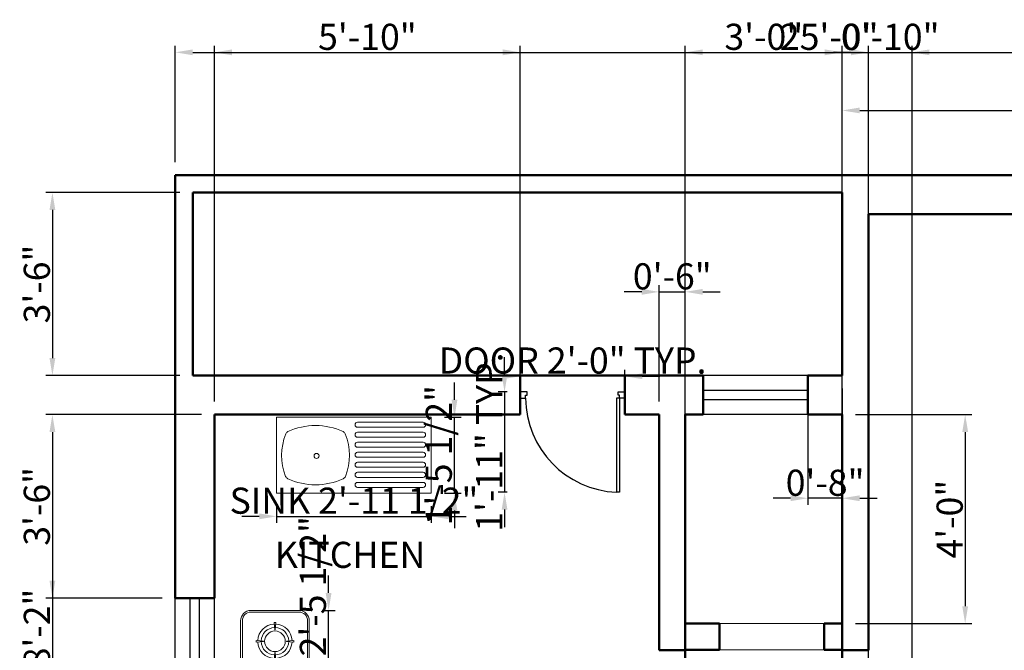
# Model space of a CAD drawing. Units: inches. Extents: x 749 to 1130, y 885 to 1490.
# Tile 4 of 5: x 754 to 980, y 1345 to 1490. Entities that reach past the tile are written whole.
import ezdxf

# ---------------------------------------------------------------- set-up
doc = ezdxf.new("R2010")
doc.units = ezdxf.units.IN
doc.header["$MEASUREMENT"] = 0
for name, color, linetype, lineweight in [('A-ANNO-DIMS', 2, 'Continuous', 18), ('A-AREA-IDEN', 7, 'Continuous', 25), ('A-DOOR', 2, 'Continuous', 25), ('A-EQPM', 8, 'Continuous', 20), ('A-FLOR-FIXT', 9, 'Continuous', 20), ('A-FLOR-OPEN', 1, 'Continuous', 18), ('WALL', 7, 'Continuous', 50), ('WINDOW', 2, 'Continuous', 25)]:
    doc.layers.add(name, color=color, linetype=linetype, lineweight=lineweight)
doc.styles.get("Standard").update_dxf_attribs({"font": 'arial.ttf'})
doc.styles.add('YQ_DIM', font='SUPEROS.SHX', dxfattribs={"width": 0.8, "bigfont": 'HZDX.SHX'})
doc.dimstyles.new('yqi0', dxfattribs={"dimscale": 0, "dimtxt": 6, "dimasz": 4, "dimexe": 1.5, "dimexo": 3, "dimgap": 0.5, "dimtad": 1, "dimdsep": 46, "dimlunit": 4, "dimtxsty": 'Standard', "dimcen": 0, "dimclrd": 256, "dimclre": 256, "dimclrt": 7, "dimadec": 1, "dimazin": 2, "dimtfac": 1, "dimtix": 1, "dimtmove": 2, "dimatfit": 2, "dimfxl": 1, "dimtolj": 1, "dimtzin": 0, "dimarcsym": 0})

# ---------------------------------------------------------------- blocks, each defined once
blk = doc.blocks.new('*D2')
at = {"layer": 'A-ANNO-DIMS', "color": 0, "lineweight": -2, "transparency": 16777216}
for p, q in [((943.07, 1457.46), (943.07, 1470.81)), ((1090.07, 1457.46), (1090.07, 1470.81)), ((947.07, 1469.31), (1086.07, 1469.31))]:
    blk.add_line(p, q, dxfattribs=at)
at = {"layer": 'A-ANNO-DIMS', "color": 0, "transparency": 16777216}
for points in [[(947.07, 1469.98), (947.07, 1468.65), (943.07, 1469.31)], [(1086.07, 1469.98), (1086.07, 1468.65), (1090.07, 1469.31)]]:
    blk.add_solid(points, dxfattribs=at)
at = {"layer": 'Defpoints', "color": 0, "transparency": 16777216}
for p in [(1090.07, 1469.31), (943.07, 1454.46), (1090.07, 1454.46)]:
    blk.add_point(p, dxfattribs=at)
at = {"layer": 'A-ANNO-DIMS', "color": 0, "transparency": 16777216, "insert": (1016.57, 1472.88), "char_height": 6, "attachment_point": 5}
blk.add_mtext('\\A1;12\'-3"', dxfattribs=at)
blk = doc.blocks.new('WD_WIN4')
for p, q in [((-0.5, 0.5), (0.5, 0.5)), ((-0.5, 0.12), (0.5, 0.12)), ((-0.5, -0.12), (0.5, -0.12)), ((-0.5, -0.5), (0.5, -0.5))]:
    blk.add_line(p, q)
blk = doc.blocks.new('DR_D01')
for p, q in [((-0.45, 0.93), (-0.42, 0.93)), ((-0.45, 0.03), (-0.45, 0.93)), ((-0.42, 0.03), (-0.42, 0.93)), ((-0.5, 0.03), (-0.42, 0.03)), ((-0.5, 0.03), (-0.5, -0.03)), ((-0.45, 0.03), (-0.45, 0)), ((-0.45, 0), (-0.435, 0)), ((-0.435, 0), (-0.435, -0.03)), ((0.435, 0), (0.435, -0.03)), ((0.45, 0), (0.435, 0)), ((0.45, 0.03), (0.45, 0)), ((0.5, 0.03), (0.45, 0.03)), ((0.5, -0.03), (0.5, 0.03)), ((-0.435, -0.03), (-0.5, -0.03)), ((0.435, -0.03), (0.5, -0.03))]:
    blk.add_line(p, q)
blk.add_arc((-0.4602, 0.0206), 0.9103, 0.59152, 87.46644)
blk = doc.blocks.new('sink7a')
for p, q in [((12297, -765), (22250, -765)), ((12297, -1527), (22250, -1527)), ((12297, -2289), (22250, -2289)), ((12297, -3051), (22250, -3051)), ((12297, -3813), (22250, -3813)), ((12297, -4575), (22250, -4575)), ((12297, -5337), (22250, -5337)), ((12297, -6099), (22250, -6099)), ((12297, -6861), (22250, -6861)), ((12297, -7623), (22250, -7623)), ((12297, -8385), (22250, -8385)), ((12297, -9147), (22250, -9147)), ((12297, -9909), (22250, -9909)), ((12297, -10671), (22250, -10671))]:
    blk.add_line(p, q)
blk.add_lwpolyline([(0, 0), (0, -11557), (23495, -11557), (23495, 0)], close=True)
blk.add_lwpolyline([(1692, -9356, -0.193356), (1368, -9011, -0.1886606), (1376, -2541, -0.1929606), (1700, -2197, -0.2205414), (10111, -2197, -0.1929606), (10435, -2541, -0.1886606), (10443, -9011, -0.193356), (10119, -9356, -0.2209789)], format="xyb", close=True)
blk.add_circle((6064, -5888), 381)
for centre, start, end in [((12297, -1146), 90, 270), ((22250, -1146), 270, 90), ((12297, -2670), 90, 270), ((22250, -2670), 270, 90), ((12297, -4194), 90, 270), ((22250, -4194), 270, 90), ((12297, -5718), 90, 270), ((22250, -5718), 270, 90), ((12297, -7242), 90, 270), ((22250, -7242), 270, 90), ((12297, -8766), 90, 270), ((22250, -8766), 270, 90), ((12297, -10290), 90, 270), ((22250, -10290), 270, 90)]:
    blk.add_arc(centre, 381, start, end)
blk = doc.blocks.new('yq_cooker_01')
for p, q in [((426.3, 34.3), (465.5, 34.3)), ((426.3, -34.3), (465.5, -34.3))]:
    blk.add_line(p, q)
for points in [[(440, -375), (160, -375, -0.414214), (100, -315), (100, 315, -0.414214), (160, 375), (440, 375, -0.414214), (500, 315), (500, -315, -0.414214)], [(440, -365), (160, -365, -0.414214), (110, -315), (110, 315, -0.414214), (160, 365), (440, 365, -0.414214), (490, 315), (490, -315, -0.414214)]]:
    blk.add_lwpolyline(points, format="xyb", close=True)
for points in [[(300.8, 261.3), (305.4, 305), (294.6, 305), (299.2, 261.3)], [(233.7, 195.8), (190, 200.4), (190, 189.6), (233.7, 194.2)], [(366.3, 194.2), (410, 189.6), (410, 200.4), (366.3, 195.8)], [(299.2, 128.7), (294.6, 85), (305.4, 85), (300.8, 128.7)], [(299.2, -128.7), (294.6, -85), (305.4, -85), (300.8, -128.7)], [(233.7, -195.8), (190, -200.4), (190, -189.6), (233.7, -194.2)], [(366.3, -194.2), (410, -189.6), (410, -200.4), (366.3, -195.8)], [(300.8, -261.3), (305.4, -305), (294.6, -305), (299.2, -261.3)]]:
    blk.add_lwpolyline(points, close=True)
blk.add_lwpolyline([(406.7, -34.3, 0.414214), (445.9, -73.5), (455.5, -73.5, 0.414214), (475.1, -53.9), (475.1, 53.9, 0.414214), (455.5, 73.5), (445.9, 73.5, 0.414214), (406.7, 34.3), (406.7, -34.3)], format="xyb")
for centre, radius in [((300, 195), 60), ((445.9, 34.3), 19.6), ((445.9, -34.3), 19.6), ((300, -195), 60)]:
    blk.add_circle(centre, radius)
for centre, radius, start, end in [((300, 195), 100, 92.4978, 177.5022), ((300, 195), 100, 2.4978, 87.5022), ((300, 195), 80, 91.59131, 178.40869), ((300, 195), 80, 1.59131, 88.40869), ((300, 195), 100, 182.4978, 267.5022), ((300, 195), 80, 181.59131, 268.40869), ((300, 195), 80, 271.59131, 358.40869), ((300, 195), 100, 272.4978, 357.5022), ((300, -195), 100, 92.4978, 177.5022), ((300, -195), 100, 2.4978, 87.5022), ((300, -195), 80, 91.59131, 178.40869), ((300, -195), 80, 1.59131, 88.40869), ((300, -195), 100, 182.4978, 267.5022), ((300, -195), 80, 181.59131, 268.40869), ((300, -195), 80, 271.59131, 358.40869), ((300, -195), 100, 272.4978, 357.5022)]:
    blk.add_arc(centre, radius, start, end)
blk = doc.blocks.new('*D19')
at = {"layer": 'A-ANNO-DIMS', "lineweight": -2, "transparency": 16777216}
for p, q in [((869.2, 1407.68), (869.2, 1409.78)), ((893.2, 1407.68), (893.2, 1409.78)), ((865.2, 1408.28), (861.2, 1408.28)), ((893.2, 1408.28), (869.2, 1408.28)), ((897.2, 1408.28), (901.2, 1408.28))]:
    blk.add_line(p, q, dxfattribs=at)
at = {"layer": 'A-ANNO-DIMS', "transparency": 16777216}
for points in [[(865.2, 1408.95), (865.2, 1407.61), (869.2, 1408.28)], [(897.2, 1408.95), (897.2, 1407.61), (893.2, 1408.28)]]:
    blk.add_solid(points, dxfattribs=at)
at = {"layer": 'Defpoints', "color": 0, "transparency": 16777216}
for p in [(869.2, 1408.28), (869.2, 1404.68), (893.2, 1404.68)]:
    blk.add_point(p, dxfattribs=at)
at = {"layer": 'A-ANNO-DIMS', "color": 7, "transparency": 16777216, "insert": (881.2, 1411.88), "char_height": 6, "attachment_point": 5}
blk.add_mtext('\\A1;DOOR 2\'-0" TYP.', dxfattribs=at)
blk = doc.blocks.new('*D20')
at = {"layer": 'A-ANNO-DIMS', "lineweight": -2, "transparency": 16777216}
for p, q in [((865.6, 1408.68), (865.6, 1412.68)), ((866.2, 1404.68), (864.1, 1404.68)), ((865.6, 1404.68), (865.6, 1381.64)), ((866.2, 1381.64), (864.1, 1381.64)), ((865.6, 1377.64), (865.6, 1373.64))]:
    blk.add_line(p, q, dxfattribs=at)
at = {"layer": 'A-ANNO-DIMS', "transparency": 16777216}
for points in [[(864.93, 1408.68), (866.26, 1408.68), (865.6, 1404.68)], [(864.93, 1377.64), (866.26, 1377.64), (865.6, 1381.64)]]:
    blk.add_solid(points, dxfattribs=at)
at = {"layer": 'Defpoints', "color": 0, "transparency": 16777216}
for p in [(869.2, 1404.68), (865.6, 1381.64), (869.2, 1381.64)]:
    blk.add_point(p, dxfattribs=at)
at = {"layer": 'A-ANNO-DIMS', "color": 7, "transparency": 16777216, "insert": (862.08, 1393.16), "char_height": 6, "attachment_point": 5, "rotation": 90}
blk.add_mtext('\\A1;1\'-11" TYP.', dxfattribs=at)
blk = doc.blocks.new('*D25')
at = {"layer": 'A-ANNO-DIMS', "lineweight": -2, "transparency": 16777216}
for p, q in [((813.31, 1378.42), (813.31, 1374.6)), ((848.79, 1378.42), (848.79, 1374.6)), ((809.31, 1376.1), (805.31, 1376.1)), ((813.31, 1376.1), (848.79, 1376.1)), ((852.79, 1376.1), (856.79, 1376.1))]:
    blk.add_line(p, q, dxfattribs=at)
at = {"layer": 'A-ANNO-DIMS', "transparency": 16777216}
for points in [[(809.31, 1376.77), (809.31, 1375.44), (813.31, 1376.1)], [(852.79, 1376.77), (852.79, 1375.44), (848.79, 1376.1)]]:
    blk.add_solid(points, dxfattribs=at)
at = {"layer": 'Defpoints', "color": 0, "transparency": 16777216}
for p in [(813.31, 1381.42), (848.79, 1381.42), (848.79, 1376.1)]:
    blk.add_point(p, dxfattribs=at)
at = {"layer": 'A-ANNO-DIMS', "color": 7, "transparency": 16777216, "insert": (831.05, 1379.7), "char_height": 6, "attachment_point": 5}
blk.add_mtext('\\A1;SINK 2\'-11 1/2"', dxfattribs=at)
blk = doc.blocks.new('*D26')
at = {"layer": 'A-ANNO-DIMS', "lineweight": -2, "transparency": 16777216}
for p, q in [((854.11, 1402.87), (854.11, 1406.87)), ((851.79, 1398.87), (855.61, 1398.87)), ((854.11, 1381.42), (854.11, 1398.87)), ((851.79, 1381.42), (855.61, 1381.42)), ((854.11, 1377.42), (854.11, 1373.42))]:
    blk.add_line(p, q, dxfattribs=at)
at = {"layer": 'A-ANNO-DIMS', "transparency": 16777216}
for points in [[(853.44, 1402.87), (854.78, 1402.87), (854.11, 1398.87)], [(853.44, 1377.42), (854.78, 1377.42), (854.11, 1381.42)]]:
    blk.add_solid(points, dxfattribs=at)
at = {"layer": 'Defpoints', "color": 0, "transparency": 16777216}
for p in [(848.79, 1398.87), (854.11, 1398.87), (848.79, 1381.42)]:
    blk.add_point(p, dxfattribs=at)
at = {"layer": 'A-ANNO-DIMS', "color": 7, "transparency": 16777216, "insert": (850.51, 1390.15), "char_height": 6, "attachment_point": 5, "rotation": 90}
blk.add_mtext('\\A1;1\'-5 1/2"', dxfattribs=at)
blk = doc.blocks.new('*D27')
at = {"layer": 'A-ANNO-DIMS', "lineweight": -2, "transparency": 16777216}
for p, q in [((825.23, 1358.5), (825.23, 1362.5)), ((823.8, 1354.5), (826.73, 1354.5)), ((825.23, 1324.97), (825.23, 1354.5)), ((823.8, 1324.97), (826.73, 1324.97)), ((825.23, 1320.97), (825.23, 1316.97))]:
    blk.add_line(p, q, dxfattribs=at)
at = {"layer": 'A-ANNO-DIMS', "transparency": 16777216}
for points in [[(824.56, 1358.5), (825.9, 1358.5), (825.23, 1354.5)], [(824.56, 1320.97), (825.9, 1320.97), (825.23, 1324.97)]]:
    blk.add_solid(points, dxfattribs=at)
at = {"layer": 'Defpoints', "color": 0, "transparency": 16777216}
for p in [(820.8, 1354.5), (825.23, 1354.5), (820.8, 1324.97)]:
    blk.add_point(p, dxfattribs=at)
at = {"layer": 'A-ANNO-DIMS', "color": 7, "transparency": 16777216, "insert": (821.63, 1339.73), "char_height": 6, "attachment_point": 5, "rotation": 90}
blk.add_mtext('\\A1;COOKTOP 2\'-5 1/2"', dxfattribs=at)
blk = doc.blocks.new('*D31')
at = {"layer": 'A-ANNO-DIMS', "lineweight": -2, "transparency": 16777216}
for p, q in [((790.07, 1457.46), (790.07, 1484.16)), ((1090.07, 1457.46), (1090.07, 1484.16)), ((794.07, 1482.66), (1086.07, 1482.66))]:
    blk.add_line(p, q, dxfattribs=at)
at = {"layer": 'A-ANNO-DIMS', "transparency": 16777216}
for points in [[(794.07, 1483.33), (794.07, 1481.99), (790.07, 1482.66)], [(1086.07, 1483.33), (1086.07, 1481.99), (1090.07, 1482.66)]]:
    blk.add_solid(points, dxfattribs=at)
at = {"layer": 'Defpoints', "color": 0, "transparency": 16777216}
for p in [(1090.07, 1482.66), (790.07, 1454.46), (1090.07, 1454.46)]:
    blk.add_point(p, dxfattribs=at)
at = {"layer": 'A-ANNO-DIMS', "color": 7, "transparency": 16777216, "insert": (940.07, 1486.22), "char_height": 6, "attachment_point": 5}
blk.add_mtext('\\A1;25\'-0"', dxfattribs=at)
blk = doc.blocks.new('*D32')
at = {"layer": 'A-ANNO-DIMS', "lineweight": -2, "transparency": 16777216}
for p, q in [((791.07, 1450.46), (760.37, 1450.46)), ((761.87, 1446.46), (761.87, 1412.46)), ((791.07, 1408.46), (760.37, 1408.46))]:
    blk.add_line(p, q, dxfattribs=at)
at = {"layer": 'A-ANNO-DIMS', "transparency": 16777216}
for points in [[(761.2, 1446.46), (762.54, 1446.46), (761.87, 1450.46)], [(761.2, 1412.46), (762.54, 1412.46), (761.87, 1408.46)]]:
    blk.add_solid(points, dxfattribs=at)
at = {"layer": 'Defpoints', "color": 0, "transparency": 16777216}
for p in [(794.07, 1450.46), (761.87, 1408.46), (794.07, 1408.46)]:
    blk.add_point(p, dxfattribs=at)
at = {"layer": 'A-ANNO-DIMS', "color": 7, "transparency": 16777216, "insert": (758.3, 1429.46), "char_height": 6, "attachment_point": 5, "rotation": 90}
blk.add_mtext('\\A1;3\'-6"', dxfattribs=at)
blk = doc.blocks.new('*D33')
at = {"layer": 'A-ANNO-DIMS', "lineweight": -2, "transparency": 16777216}
for p, q in [((796.07, 1399.46), (760.37, 1399.46)), ((761.87, 1395.46), (761.87, 1305.46)), ((796.07, 1301.46), (760.37, 1301.46))]:
    blk.add_line(p, q, dxfattribs=at)
at = {"layer": 'A-ANNO-DIMS', "transparency": 16777216}
for points in [[(761.2, 1395.46), (762.54, 1395.46), (761.87, 1399.46)], [(761.2, 1305.46), (762.54, 1305.46), (761.87, 1301.46)]]:
    blk.add_solid(points, dxfattribs=at)
at = {"layer": 'Defpoints', "color": 0, "transparency": 16777216}
for p in [(799.07, 1399.46), (761.87, 1301.46), (799.07, 1301.46)]:
    blk.add_point(p, dxfattribs=at)
at = {"layer": 'A-ANNO-DIMS', "color": 7, "transparency": 16777216, "insert": (758.31, 1350.46), "char_height": 6, "attachment_point": 5, "rotation": 90}
blk.add_mtext('\\A1;8\'-2"', dxfattribs=at)
blk = doc.blocks.new('*D42')
at = {"layer": 'A-ANNO-DIMS', "lineweight": -2, "transparency": 16777216}
for p, q in [((907.07, 1354.46), (907.07, 1484.16)), ((943.07, 1354.46), (943.07, 1484.16)), ((911.07, 1482.66), (939.07, 1482.66))]:
    blk.add_line(p, q, dxfattribs=at)
at = {"layer": 'A-ANNO-DIMS', "transparency": 16777216}
for points in [[(911.07, 1483.33), (911.07, 1481.99), (907.07, 1482.66)], [(939.07, 1483.33), (939.07, 1481.99), (943.07, 1482.66)]]:
    blk.add_solid(points, dxfattribs=at)
at = {"layer": 'Defpoints', "color": 0, "transparency": 16777216}
for p in [(943.07, 1482.66), (907.07, 1351.46), (943.07, 1351.46)]:
    blk.add_point(p, dxfattribs=at)
at = {"layer": 'A-ANNO-DIMS', "color": 7, "transparency": 16777216, "insert": (925.07, 1486.23), "char_height": 6, "attachment_point": 5}
blk.add_mtext('\\A1;3\'-0"', dxfattribs=at)
blk = doc.blocks.new('*D43')
at = {"layer": 'A-ANNO-DIMS', "lineweight": -2, "transparency": 16777216}
for p, q in [((799.07, 1402.46), (799.07, 1484.16)), ((869.2, 1402.46), (869.2, 1484.16)), ((803.07, 1482.66), (865.2, 1482.66))]:
    blk.add_line(p, q, dxfattribs=at)
at = {"layer": 'A-ANNO-DIMS', "transparency": 16777216}
for points in [[(803.07, 1483.33), (803.07, 1481.99), (799.07, 1482.66)], [(865.2, 1483.33), (865.2, 1481.99), (869.2, 1482.66)]]:
    blk.add_solid(points, dxfattribs=at)
at = {"layer": 'Defpoints', "color": 0, "transparency": 16777216}
for p in [(869.2, 1482.66), (799.07, 1399.46), (869.2, 1399.46)]:
    blk.add_point(p, dxfattribs=at)
at = {"layer": 'A-ANNO-DIMS', "color": 7, "transparency": 16777216, "insert": (834.13, 1486.22), "char_height": 6, "attachment_point": 5}
blk.add_mtext('\\A1;5\'-10"', dxfattribs=at)
blk = doc.blocks.new('*D44')
at = {"layer": 'A-ANNO-DIMS', "lineweight": -2, "transparency": 16777216}
for p, q in [((796.07, 1399.46), (760.37, 1399.46)), ((761.87, 1395.46), (761.87, 1361.33)), ((787.07, 1357.33), (760.37, 1357.33))]:
    blk.add_line(p, q, dxfattribs=at)
at = {"layer": 'A-ANNO-DIMS', "transparency": 16777216}
for points in [[(761.2, 1395.46), (762.54, 1395.46), (761.87, 1399.46)], [(761.2, 1361.33), (762.54, 1361.33), (761.87, 1357.33)]]:
    blk.add_solid(points, dxfattribs=at)
at = {"layer": 'Defpoints', "color": 0, "transparency": 16777216}
for p in [(799.07, 1399.46), (761.87, 1357.33), (790.07, 1357.33)]:
    blk.add_point(p, dxfattribs=at)
at = {"layer": 'A-ANNO-DIMS', "color": 7, "transparency": 16777216, "insert": (758.3, 1378.4), "char_height": 6, "attachment_point": 5, "rotation": 90}
blk.add_mtext('\\A1;3\'-6"', dxfattribs=at)
blk = doc.blocks.new('*D47')
at = {"layer": 'A-ANNO-DIMS', "lineweight": -2, "transparency": 16777216}
for p, q in [((949.07, 1087.46), (949.07, 1484.16)), ((959.07, 1087.46), (959.07, 1484.16)), ((945.07, 1482.66), (941.07, 1482.66)), ((949.07, 1482.66), (959.07, 1482.66)), ((963.07, 1482.66), (967.07, 1482.66))]:
    blk.add_line(p, q, dxfattribs=at)
at = {"layer": 'A-ANNO-DIMS', "transparency": 16777216}
for points in [[(945.07, 1483.33), (945.07, 1481.99), (949.07, 1482.66)], [(963.07, 1483.33), (963.07, 1481.99), (959.07, 1482.66)]]:
    blk.add_solid(points, dxfattribs=at)
at = {"layer": 'Defpoints', "color": 0, "transparency": 16777216}
for p in [(959.07, 1482.66), (949.07, 1084.46), (959.07, 1084.46)]:
    blk.add_point(p, dxfattribs=at)
at = {"layer": 'A-ANNO-DIMS', "color": 7, "transparency": 16777216, "insert": (954.07, 1486.22), "char_height": 6, "attachment_point": 5}
blk.add_mtext('\\A1;0\'-10"', dxfattribs=at)
blk = doc.blocks.new('*D57')
at = {"layer": 'A-ANNO-DIMS', "lineweight": -2, "transparency": 16777216}
for p, q in [((946.07, 1399.46), (972.77, 1399.46)), ((971.27, 1395.46), (971.27, 1355.46)), ((946.07, 1351.46), (972.77, 1351.46))]:
    blk.add_line(p, q, dxfattribs=at)
at = {"layer": 'A-ANNO-DIMS', "transparency": 16777216}
for points in [[(970.6, 1395.46), (971.94, 1395.46), (971.27, 1399.46)], [(970.6, 1355.46), (971.94, 1355.46), (971.27, 1351.46)]]:
    blk.add_solid(points, dxfattribs=at)
at = {"layer": 'Defpoints', "color": 0, "transparency": 16777216}
for p in [(943.07, 1399.46), (943.07, 1351.46), (971.27, 1351.46)]:
    blk.add_point(p, dxfattribs=at)
at = {"layer": 'A-ANNO-DIMS', "color": 7, "transparency": 16777216, "insert": (967.71, 1375.46), "char_height": 6, "attachment_point": 5, "rotation": 90}
blk.add_mtext('\\A1;4\'-0"', dxfattribs=at)
blk = doc.blocks.new('*D66')
at = {"layer": 'A-ANNO-DIMS', "lineweight": -2, "transparency": 16777216}
for p, q in [((935.2, 1405.46), (935.2, 1378.76)), ((943.07, 1405.46), (943.07, 1378.76)), ((931.2, 1380.26), (927.2, 1380.26)), ((943.07, 1380.26), (935.2, 1380.26)), ((947.07, 1380.26), (951.07, 1380.26))]:
    blk.add_line(p, q, dxfattribs=at)
at = {"layer": 'A-ANNO-DIMS', "transparency": 16777216}
for points in [[(931.2, 1380.93), (931.2, 1379.59), (935.2, 1380.26)], [(947.07, 1380.93), (947.07, 1379.59), (943.07, 1380.26)]]:
    blk.add_solid(points, dxfattribs=at)
at = {"layer": 'Defpoints', "color": 0, "transparency": 16777216}
for p in [(935.2, 1408.46), (943.07, 1408.46), (935.2, 1380.26)]:
    blk.add_point(p, dxfattribs=at)
at = {"layer": 'A-ANNO-DIMS', "color": 7, "transparency": 16777216, "insert": (939.13, 1383.82), "char_height": 6, "attachment_point": 5}
blk.add_mtext('\\A1;0\'-8"', dxfattribs=at)
blk = doc.blocks.new('*D67')
at = {"layer": 'A-ANNO-DIMS', "lineweight": -2, "transparency": 16777216}
for p, q in [((897.07, 1427.66), (893.07, 1427.66)), ((901.07, 1402.46), (901.07, 1429.16)), ((901.07, 1427.66), (907.07, 1427.66)), ((907.07, 1402.46), (907.07, 1429.16)), ((911.07, 1427.66), (915.07, 1427.66))]:
    blk.add_line(p, q, dxfattribs=at)
at = {"layer": 'A-ANNO-DIMS', "transparency": 16777216}
for points in [[(897.07, 1428.33), (897.07, 1426.99), (901.07, 1427.66)], [(911.07, 1428.33), (911.07, 1426.99), (907.07, 1427.66)]]:
    blk.add_solid(points, dxfattribs=at)
at = {"layer": 'Defpoints', "color": 0, "transparency": 16777216}
for p in [(907.07, 1427.66), (901.07, 1399.46), (907.07, 1399.46)]:
    blk.add_point(p, dxfattribs=at)
at = {"layer": 'A-ANNO-DIMS', "color": 7, "transparency": 16777216, "insert": (904.07, 1431.22), "char_height": 6, "attachment_point": 5}
blk.add_mtext('\\A1;0\'-6"', dxfattribs=at)

msp = doc.modelspace()

# ---------------------------------------------------------------- linework, layer by layer
at = {"layer": 'A-FLOR-OPEN'}
for p, q in [((914.944, 1351.46), (938.944, 1351.46)), ((914.944, 1345.46), (938.944, 1345.46))]:
    msp.add_line(p, q, dxfattribs=at)
at = {"layer": 'WALL'}
for p, q in [((943.07, 1454.46), (790.07, 1454.46)), ((790.07, 1450.46), (790.07, 1454.46)), ((943.07, 1454.46), (1090.07, 1454.46)), ((790.07, 1450.46), (790.07, 1408.46)), ((943.07, 1450.46), (794.07, 1450.46)), ((794.07, 1450.46), (794.07, 1408.46)), ((943.07, 1408.46), (943.07, 1450.46)), ((949.07, 1445.46), (1081.07, 1445.46)), ((949.07, 1345.334), (949.07, 1445.46)), ((790.07, 1357.334), (790.07, 1408.46)), ((794.07, 1408.46), (893.196, 1408.46)), ((869.196, 1399.46), (869.196, 1408.46)), ((893.196, 1408.46), (911.196, 1408.46)), ((893.196, 1399.46), (893.196, 1408.46)), ((911.196, 1399.46), (911.196, 1408.46)), ((935.196, 1408.46), (943.07, 1408.46)), ((935.196, 1399.46), (935.196, 1408.46)), ((799.07, 1399.46), (869.196, 1399.46)), ((799.07, 1357.334), (799.07, 1399.46)), ((893.196, 1399.46), (901.07, 1399.46)), ((901.07, 1345.334), (901.07, 1399.46)), ((907.07, 1399.46), (911.196, 1399.46)), ((907.07, 1351.46), (907.07, 1399.46)), ((935.196, 1399.46), (943.07, 1399.46)), ((943.07, 1309.334), (943.07, 1399.46)), ((799.07, 1357.334), (790.07, 1357.334)), ((907.07, 1351.46), (914.944, 1351.46)), ((907.07, 1345.334), (907.07, 1351.46)), ((914.944, 1351.46), (914.944, 1345.46)), ((938.944, 1351.46), (943.07, 1351.46)), ((938.944, 1351.46), (938.944, 1345.46)), ((901.07, 1345.334), (907.07, 1345.334)), ((907.07, 1345.46), (914.944, 1345.46)), ((907.07, 1295.46), (907.07, 1345.334)), ((938.944, 1345.46), (943.07, 1345.46)), ((943.07, 1345.334), (943.07, 1345.46)), ((949.07, 1345.334), (943.07, 1345.334))]:
    msp.add_line(p, q, dxfattribs=at)

# ---------------------------------------------------------------- block references
at = {"layer": 'A-DOOR', "xscale": 24, "yscale": 24, "zscale": 24, "rotation": 180}
msp.add_blockref('DR_D01', (881.196, 1403.96), dxfattribs=at)
at = {"layer": 'A-EQPM', "xscale": 0.0393700787401575, "yscale": 0.0393700787401575, "zscale": 0.0393700787401575}
msp.add_blockref('yq_cooker_01', (801.117, 1339.735), dxfattribs=at)
at = {"layer": 'A-FLOR-FIXT', "xscale": 0.0015098735489763, "yscale": 0.0015098735489763, "zscale": 0.0015098735489763}
msp.add_blockref('sink7a', (813.315, 1398.873), dxfattribs=at)
at = {"layer": 'WINDOW'}
for p, xscale, yscale, zscale, rotation in [((923.196, 1403.96), 24, 9.000000000000227, 24, 180.0000000000005), ((794.57, 1333.334), 48, 8.999999999998522, 48, 89.99999999999973)]:
    msp.add_blockref('WD_WIN4', p, dxfattribs=dict(at, xscale=xscale, yscale=yscale, zscale=zscale, rotation=rotation))

# ---------------------------------------------------------------- texts
at = {"layer": 'A-AREA-IDEN', "insert": (810.318, 1370.258), "char_height": 13.77953, "width": 39.68725, "attachment_point": 1, "style": 'YQ_DIM'}
msp.add_mtext('\\pxqc;{\\H0.43543x;KITCHEN}', dxfattribs=at)

# ---------------------------------------------------------------- dimensions: what is measured, and where the dimension line sits
at = {"layer": 'A-ANNO-DIMS'}
for base, p1, p2, picture, middle in [((1090.07, 1482.66), (790.07, 1454.46), (1090.07, 1454.46), '*D31', (940.07, 1486.224)), ((869.196, 1482.66), (799.07, 1399.46), (869.196, 1399.46), '*D43', (834.133, 1486.224)), ((943.07, 1482.66), (907.07, 1351.46), (943.07, 1351.46), '*D42', (925.07, 1486.226)), ((959.07, 1482.66), (949.07, 1084.46), (959.07, 1084.46), '*D47', (954.07, 1486.224)), ((907.07, 1427.66), (901.07, 1399.46), (907.07, 1399.46), '*D67', (904.07, 1431.224))]:
    dim = msp.add_linear_dim(base=base, p1=p1, p2=p2, dimstyle='yqi0', override={"dimscale": 1, "dimdec": 1, "dimzin": 1, "dimfrac": 2}, dxfattribs=at)
    dim.commit()
    dim.dimension.update_dxf_attribs({"geometry": picture, "text_midpoint": middle})
dim = msp.add_aligned_dim(p1=(943.07, 1454.46), p2=(1090.07, 1454.46), distance=14.854, dimstyle='yqi0', override={"dimscale": 1, "dimclrd": 0, "dimclre": 0, "dimclrt": 0}, dxfattribs=at)
dim.commit()
dim.dimension.update_dxf_attribs({"geometry": '*D2', "text_midpoint": (1016.57, 1472.88)})
for base, p1, p2, angle, picture, middle in [((761.87, 1408.46), (794.07, 1450.46), (794.07, 1408.46), 90, '*D32', (758.304, 1429.46)), ((935.196, 1380.26), (943.07, 1408.46), (935.196, 1408.46), 180, '*D66', (939.133, 1383.824)), ((854.111, 1398.873), (848.789, 1381.424), (848.789, 1398.873), 90, '*D26', (850.508, 1390.148)), ((761.87, 1357.334), (799.07, 1399.46), (790.07, 1357.334), 90, '*D44', (758.304, 1378.397)), ((761.87, 1301.46), (799.07, 1399.46), (799.07, 1301.46), 90, '*D33', (758.306, 1350.46)), ((971.27, 1351.46), (943.07, 1399.46), (943.07, 1351.46), 270, '*D57', (967.706, 1375.46))]:
    dim = msp.add_linear_dim(base=base, p1=p1, p2=p2, angle=angle, dimstyle='yqi0', override={"dimscale": 1, "dimdec": 1, "dimzin": 1, "dimfrac": 2}, dxfattribs=at)
    dim.commit()
    dim.dimension.update_dxf_attribs({"geometry": picture, "text_midpoint": middle})
for base, p1, p2, angle, text, picture, middle in [((869.196, 1408.28), (893.196, 1404.68), (869.196, 1404.68), 180, 'DOOR <> TYP.', '*D19', (881.196, 1411.885)), ((865.596, 1381.64), (869.196, 1404.68), (869.196, 1381.64), 270, '<> TYP.', '*D20', (862.082, 1393.16)), ((825.231, 1354.498), (820.802, 1324.971), (820.802, 1354.498), 90, 'COOKTOP <>', '*D27', (821.627, 1339.735))]:
    dim = msp.add_linear_dim(base=base, p1=p1, p2=p2, angle=angle, text=text, dimstyle='yqi0', override={"dimscale": 1, "dimdec": 1, "dimzin": 1, "dimfrac": 2}, dxfattribs=at)
    dim.commit()
    dim.dimension.update_dxf_attribs({"geometry": picture, "text_midpoint": middle})
dim = msp.add_linear_dim(base=(848.789, 1376.102), p1=(813.315, 1381.424), p2=(848.789, 1381.424), text='SINK <>', dimstyle='yqi0', override={"dimscale": 1, "dimdec": 1, "dimzin": 1, "dimfrac": 2}, dxfattribs=at)
dim.commit()
dim.dimension.update_dxf_attribs({"geometry": '*D25', "text_midpoint": (831.052, 1379.705)})

doc.saveas('drawing.dxf')
